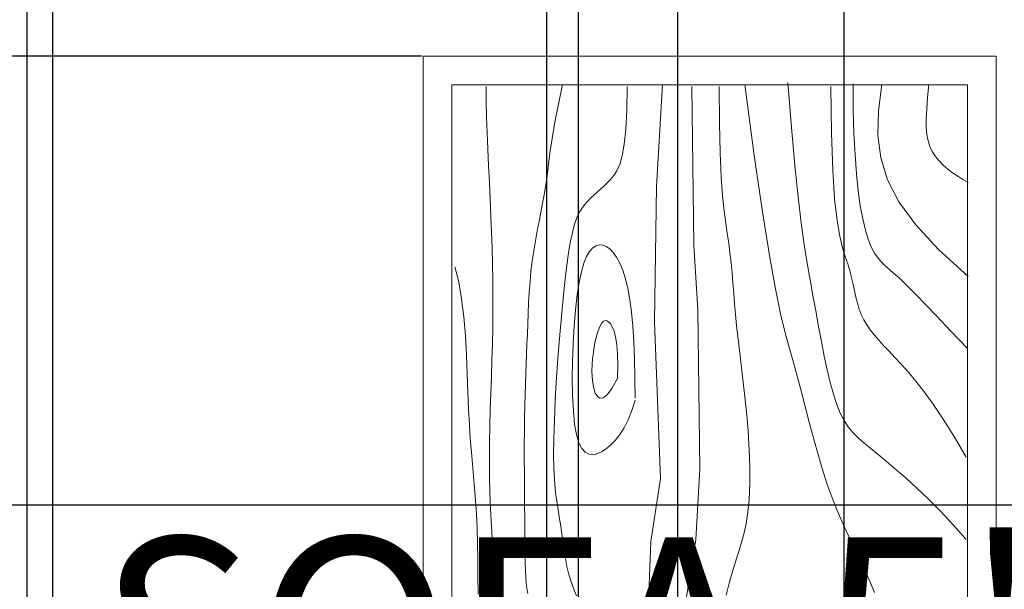
# Model space of a CAD drawing. Units: inches. Extents: x -26 to 385, y 12 to 697.
# Tile 7 of 13: x 223 to 264, y 191 to 215. Entities that reach past the tile are written whole.
import ezdxf

# ---------------------------------------------------------------- set-up
doc = ezdxf.new("R2010")
doc.units = ezdxf.units.IN
doc.header["$MEASUREMENT"] = 0
doc.layers.add('A-ANNO-DIMS', color=4, linetype='Continuous', lineweight=18)
doc.layers.add('Furniture', color=210, linetype='Continuous', lineweight=15)
doc.styles.get("Standard").update_dxf_attribs({"font": 'italic8.shx'})
doc.dimstyles.get("Standard").update_dxf_attribs({"dimtxt": 8, "dimasz": 0.18, "dimexe": 0.18, "dimexo": 0.0625, "dimgap": 0.09, "dimtad": 0, "dimtih": 1, "dimtoh": 1, "dimdec": 4, "dimzin": 0, "dimdsep": 46, "dimlunit": 3, "dimtxsty": 'Standard', "dimcen": 0.09, "dimclrd": 2, "dimclre": 3, "dimclrt": 6, "dimadec": 0, "dimazin": 0, "dimtfac": 1, "dimtdec": 4, "dimtofl": 0, "dimtmove": 0, "dimatfit": 3, "dimfxl": 1, "dimtolj": 1, "dimtzin": 0, "dimarcsym": 0})

# ---------------------------------------------------------------- blocks, each defined once
blk = doc.blocks.new('*D11')
at = {"layer": 'A-ANNO-DIMS', "color": 3, "lineweight": -2, "transparency": 16777216}
for p, q in [((285.56, 224.402), (274.992, 224.402)), ((285.56, 154.738), (274.992, 154.738))]:
    blk.add_line(p, q, dxfattribs=at)
at = {"layer": 'A-ANNO-DIMS', "color": 2, "lineweight": -2, "transparency": 16777216}
for p, q in [((275.172, 224.222), (275.172, 195.755)), ((275.172, 154.918), (275.172, 183.384))]:
    blk.add_line(p, q, dxfattribs=at)
at = {"layer": 'A-ANNO-DIMS', "color": 2, "transparency": 16777216}
for points in [[(275.142, 224.222), (275.202, 224.222), (275.172, 224.402)], [(275.142, 154.918), (275.202, 154.918), (275.172, 154.738)]]:
    blk.add_solid(points, dxfattribs=at)
at = {"layer": 'Defpoints', "color": 0, "transparency": 16777216}
for p in [(285.622, 224.402), (275.172, 154.738), (285.622, 154.738)]:
    blk.add_point(p, dxfattribs=at)
at = {"layer": 'A-ANNO-DIMS', "color": 6, "transparency": 16777216, "insert": (275.172, 189.57), "char_height": 8, "attachment_point": 5}
blk.add_mtext('\\A1;SOFA 5\'-9 1/2" TYP.', dxfattribs=at)
blk = doc.blocks.new('*D28')
at = {"layer": 'A-ANNO-DIMS', "color": 3, "lineweight": -2, "transparency": 16777216}
for p, q in [((141.692, 194.903), (355.559, 194.903)), ((141.692, 158.903), (355.559, 158.903))]:
    blk.add_line(p, q, dxfattribs=at)
at = {"layer": 'A-ANNO-DIMS', "color": 2, "lineweight": -2, "transparency": 16777216}
for p, q in [((355.379, 194.723), (355.379, 181.755)), ((355.379, 159.083), (355.379, 172.052))]:
    blk.add_line(p, q, dxfattribs=at)
at = {"layer": 'A-ANNO-DIMS', "color": 2, "transparency": 16777216}
for points in [[(355.349, 194.723), (355.409, 194.723), (355.379, 194.903)], [(355.349, 159.083), (355.409, 159.083), (355.379, 158.903)]]:
    blk.add_solid(points, dxfattribs=at)
at = {"layer": 'Defpoints', "color": 0, "transparency": 16777216}
for p in [(141.629, 194.903), (355.379, 194.903), (141.629, 158.903)]:
    blk.add_point(p, dxfattribs=at)
at = {"layer": 'A-ANNO-DIMS', "color": 6, "transparency": 16777216, "insert": (355.379, 176.903), "char_height": 8, "attachment_point": 5}
blk.add_mtext('\\A1;3\'-0"', dxfattribs=at)
blk = doc.blocks.new('*D32')
at = {"layer": 'A-ANNO-DIMS', "color": 3, "lineweight": -2, "transparency": 16777216}
for p, q in [((239.825, 213.385), (-5.301, 213.385)), ((239.825, 166.141), (-5.301, 166.141))]:
    blk.add_line(p, q, dxfattribs=at)
at = {"layer": 'A-ANNO-DIMS', "color": 2, "lineweight": -2, "transparency": 16777216}
for p, q in [((-5.121, 213.205), (-5.121, 194.615)), ((-5.121, 166.321), (-5.121, 184.911))]:
    blk.add_line(p, q, dxfattribs=at)
at = {"layer": 'A-ANNO-DIMS', "color": 2, "transparency": 16777216}
for points in [[(-5.151, 213.205), (-5.091, 213.205), (-5.121, 213.385)], [(-5.151, 166.321), (-5.091, 166.321), (-5.121, 166.141)]]:
    blk.add_solid(points, dxfattribs=at)
at = {"layer": 'Defpoints', "color": 0, "transparency": 16777216}
for p in [(-5.121, 213.385), (239.888, 213.385), (239.888, 166.141)]:
    blk.add_point(p, dxfattribs=at)
at = {"layer": 'A-ANNO-DIMS', "color": 6, "transparency": 16777216, "insert": (-5.121, 189.763), "char_height": 8, "attachment_point": 5}
blk.add_mtext('\\A1;3\'-11"', dxfattribs=at)
blk = doc.blocks.new('*D35')
at = {"layer": 'A-ANNO-DIMS', "color": 3, "lineweight": -2, "transparency": 16777216}
for p, q in [((193.598, 147.942), (193.598, 684.809)), ((244.986, 147.942), (244.986, 684.809))]:
    blk.add_line(p, q, dxfattribs=at)
at = {"layer": 'A-ANNO-DIMS', "color": 2, "lineweight": -2, "transparency": 16777216}
for p, q in [((193.778, 684.629), (244.806, 684.629)), ((244.986, 684.629), (245.166, 684.629))]:
    blk.add_line(p, q, dxfattribs=at)
at = {"layer": 'A-ANNO-DIMS', "color": 2, "transparency": 16777216}
for points in [[(193.778, 684.659), (193.778, 684.599), (193.598, 684.629)], [(244.806, 684.659), (244.806, 684.599), (244.986, 684.629)]]:
    blk.add_solid(points, dxfattribs=at)
at = {"layer": 'Defpoints', "color": 0, "transparency": 16777216}
for p in [(244.986, 684.629), (193.598, 147.879), (244.986, 147.879)]:
    blk.add_point(p, dxfattribs=at)
at = {"layer": 'A-ANNO-DIMS', "color": 6, "transparency": 16777216, "insert": (278.398, 684.629), "char_height": 8, "attachment_point": 5}
blk.add_mtext('\\A1;4\'-3 1/2"', dxfattribs=at)
blk = doc.blocks.new('*D36')
at = {"layer": 'A-ANNO-DIMS', "color": 3, "lineweight": -2, "transparency": 16777216}
for p, q in [((146.129, 147.942), (146.129, 684.809)), ((193.598, 147.942), (193.598, 684.809))]:
    blk.add_line(p, q, dxfattribs=at)
at = {"layer": 'A-ANNO-DIMS', "color": 2, "lineweight": -2, "transparency": 16777216}
for p, q in [((146.309, 684.629), (193.418, 684.629)), ((193.598, 684.629), (193.778, 684.629))]:
    blk.add_line(p, q, dxfattribs=at)
at = {"layer": 'A-ANNO-DIMS', "color": 2, "transparency": 16777216}
for points in [[(146.309, 684.659), (146.309, 684.599), (146.129, 684.629)], [(193.418, 684.659), (193.418, 684.599), (193.598, 684.629)]]:
    blk.add_solid(points, dxfattribs=at)
at = {"layer": 'Defpoints', "color": 0, "transparency": 16777216}
for p in [(193.598, 684.629), (146.129, 147.879), (193.598, 147.879)]:
    blk.add_point(p, dxfattribs=at)
at = {"layer": 'A-ANNO-DIMS', "color": 6, "transparency": 16777216, "insert": (228.344, 684.629), "char_height": 8, "attachment_point": 5}
blk.add_mtext('\\A1;3\'-11 1/2"', dxfattribs=at)
blk = doc.blocks.new('*D37')
at = {"layer": 'A-ANNO-DIMS', "color": 3, "lineweight": -2, "transparency": 16777216}
for p, q in [((223.549, 597.317), (223.549, 23.949)), ((257.22, 597.317), (257.22, 23.949))]:
    blk.add_line(p, q, dxfattribs=at)
at = {"layer": 'A-ANNO-DIMS', "color": 2, "lineweight": -2, "transparency": 16777216}
for p, q in [((223.729, 24.129), (257.04, 24.129)), ((257.22, 24.129), (257.4, 24.129))]:
    blk.add_line(p, q, dxfattribs=at)
at = {"layer": 'A-ANNO-DIMS', "color": 2, "transparency": 16777216}
for points in [[(223.729, 24.159), (223.729, 24.099), (223.549, 24.129)], [(257.04, 24.159), (257.04, 24.099), (257.22, 24.129)]]:
    blk.add_solid(points, dxfattribs=at)
at = {"layer": 'Defpoints', "color": 0, "transparency": 16777216}
for p in [(223.549, 597.379), (257.22, 597.379), (257.22, 24.129)]:
    blk.add_point(p, dxfattribs=at)
at = {"layer": 'A-ANNO-DIMS', "color": 6, "transparency": 16777216, "insert": (290.633, 24.129), "char_height": 8, "attachment_point": 5}
blk.add_mtext('\\A1;2\'-9 1/2"', dxfattribs=at)
blk = doc.blocks.new('*D39')
at = {"layer": 'A-ANNO-DIMS', "color": 3, "lineweight": -2, "transparency": 16777216}
for p, q in [((183.359, 597.317), (183.359, 23.949)), ((213.359, 597.317), (213.359, 23.949))]:
    blk.add_line(p, q, dxfattribs=at)
at = {"layer": 'A-ANNO-DIMS', "color": 2, "lineweight": -2, "transparency": 16777216}
for p, q in [((183.539, 24.129), (213.179, 24.129)), ((213.359, 24.129), (213.539, 24.129))]:
    blk.add_line(p, q, dxfattribs=at)
at = {"layer": 'A-ANNO-DIMS', "color": 2, "transparency": 16777216}
for points in [[(183.539, 24.159), (183.539, 24.099), (183.359, 24.129)], [(213.179, 24.159), (213.179, 24.099), (213.359, 24.129)]]:
    blk.add_solid(points, dxfattribs=at)
at = {"layer": 'Defpoints', "color": 0, "transparency": 16777216}
for p in [(183.359, 597.379), (213.359, 597.379), (213.359, 24.129)]:
    blk.add_point(p, dxfattribs=at)
at = {"layer": 'A-ANNO-DIMS', "color": 6, "transparency": 16777216, "insert": (231.533, 24.129), "char_height": 8, "attachment_point": 5}
blk.add_mtext('\\A1;2\'-6"', dxfattribs=at)
blk = doc.blocks.new('*D42')
at = {"layer": 'A-ANNO-DIMS', "color": 3, "lineweight": -2, "transparency": 16777216}
for p, q in [((250.371, 518.992), (250.371, 23.949)), ((274.129, 518.992), (274.129, 23.949))]:
    blk.add_line(p, q, dxfattribs=at)
at = {"layer": 'A-ANNO-DIMS', "color": 2, "lineweight": -2, "transparency": 16777216}
for p, q in [((250.551, 24.129), (273.949, 24.129)), ((274.129, 24.129), (274.309, 24.129))]:
    blk.add_line(p, q, dxfattribs=at)
at = {"layer": 'A-ANNO-DIMS', "color": 2, "transparency": 16777216}
for points in [[(250.551, 24.159), (250.551, 24.099), (250.371, 24.129)], [(273.949, 24.159), (273.949, 24.099), (274.129, 24.129)]]:
    blk.add_solid(points, dxfattribs=at)
at = {"layer": 'Defpoints', "color": 0, "transparency": 16777216}
for p in [(250.371, 519.055), (274.129, 519.055), (274.129, 24.129)]:
    blk.add_point(p, dxfattribs=at)
at = {"layer": 'A-ANNO-DIMS', "color": 6, "transparency": 16777216, "insert": (292.304, 24.129), "char_height": 8, "attachment_point": 5}
blk.add_mtext('\\A1;2\'-0"', dxfattribs=at)
blk = doc.blocks.new('*D46')
at = {"layer": 'A-ANNO-DIMS', "color": 3, "lineweight": -2, "transparency": 16777216}
for p, q in [((224.595, 477.317), (224.595, 23.949)), ((284.629, 477.317), (284.629, 23.949))]:
    blk.add_line(p, q, dxfattribs=at)
at = {"layer": 'A-ANNO-DIMS', "color": 2, "lineweight": -2, "transparency": 16777216}
for p, q in [((224.775, 24.129), (236.617, 24.129)), ((284.449, 24.129), (272.607, 24.129))]:
    blk.add_line(p, q, dxfattribs=at)
at = {"layer": 'A-ANNO-DIMS', "color": 2, "transparency": 16777216}
for points in [[(224.775, 24.159), (224.775, 24.099), (224.595, 24.129)], [(284.449, 24.159), (284.449, 24.099), (284.629, 24.129)]]:
    blk.add_solid(points, dxfattribs=at)
at = {"layer": 'Defpoints', "color": 0, "transparency": 16777216}
for p in [(224.595, 477.379), (284.629, 477.379), (284.629, 24.129)]:
    blk.add_point(p, dxfattribs=at)
at = {"layer": 'A-ANNO-DIMS', "color": 6, "transparency": 16777216, "insert": (254.612, 24.129), "char_height": 8, "attachment_point": 5}
blk.add_mtext('\\A1;5\'-0"', dxfattribs=at)
blk = doc.blocks.new('*D50')
at = {"layer": 'A-ANNO-DIMS', "color": 3, "lineweight": -2, "transparency": 16777216}
for p, q in [((246.278, 401.871), (246.278, 23.949)), ((284.629, 398.317), (284.629, 23.949))]:
    blk.add_line(p, q, dxfattribs=at)
at = {"layer": 'A-ANNO-DIMS', "color": 2, "lineweight": -2, "transparency": 16777216}
for p, q in [((246.458, 24.129), (284.449, 24.129)), ((284.629, 24.129), (284.809, 24.129))]:
    blk.add_line(p, q, dxfattribs=at)
at = {"layer": 'A-ANNO-DIMS', "color": 2, "transparency": 16777216}
for points in [[(246.458, 24.159), (246.458, 24.099), (246.278, 24.129)], [(284.449, 24.159), (284.449, 24.099), (284.629, 24.129)]]:
    blk.add_solid(points, dxfattribs=at)
at = {"layer": 'Defpoints', "color": 0, "transparency": 16777216}
for p in [(246.278, 401.934), (284.629, 398.379), (284.629, 24.129)]:
    blk.add_point(p, dxfattribs=at)
at = {"layer": 'A-ANNO-DIMS', "color": 6, "transparency": 16777216, "insert": (318.042, 24.129), "char_height": 8, "attachment_point": 5}
blk.add_mtext('\\A1;3\'-2 1/2"', dxfattribs=at)

msp = doc.modelspace()

# ---------------------------------------------------------------- linework, layer by layer
at = {"layer": 'Furniture'}
for p, q in [((239.88756, 166.14113), (239.88756, 213.38513)), ((239.88756, 213.38513), (263.50956, 213.38513)), ((263.50956, 213.38513), (263.50956, 166.14113)), ((254.91435, 212.30259), (255.06209, 210.44149)), ((241.06866, 167.32223), (241.06866, 212.20403)), ((241.06866, 212.20403), (262.32846, 212.20403)), ((242.4795, 212.14102), (242.48485, 211.52259)), ((245.62858, 212.2218), (245.44175, 211.33552)), ((248.29319, 212.14102), (248.27861, 211.15771)), ((249.74662, 212.2218), (249.50438, 208.0209)), ((250.9578, 212.14102), (251.03855, 205.5973)), ((252.08825, 212.14102), (252.09894, 210.63069)), ((253.13794, 212.2218), (253.53101, 209.28852)), ((256.69075, 212.14102), (256.71032, 210.21153)), ((257.60587, 212.24873), (257.61514, 211.18493)), ((258.79014, 212.2218), (258.65467, 211.12945)), ((260.72804, 212.2218), (260.67533, 211.68458)), ((262.32846, 212.20403), (262.32846, 167.32223)), ((242.48485, 211.52259), (242.49958, 210.88199)), ((260.67533, 211.68458), (260.63941, 211.2186)), ((245.44175, 211.33552), (245.29971, 210.59976)), ((248.27861, 211.15771), (248.23705, 210.37139)), ((257.61514, 211.18493), (257.64215, 210.21382)), ((258.65467, 211.12945), (258.62991, 210.13271)), ((260.63941, 211.2186), (260.62195, 210.81557)), ((242.49958, 210.88199), (242.52172, 210.22356)), ((260.62195, 210.81557), (260.62459, 210.46722)), ((245.29971, 210.59976), (245.19426, 209.99086)), ((248.23705, 210.37139), (248.17184, 209.75564)), ((252.09894, 210.63069), (252.12841, 209.40437)), ((255.06209, 210.44149), (255.20306, 208.88799)), ((260.62459, 210.46722), (260.64899, 210.16526)), ((242.52172, 210.22356), (242.54931, 209.55164)), ((245.19426, 209.99086), (245.11719, 209.48516)), ((256.71032, 210.21153), (256.76404, 208.68676)), ((257.64215, 210.21382), (257.68571, 209.33343)), ((258.62991, 210.13271), (258.74331, 209.19846)), ((260.64899, 210.16526), (260.69682, 209.9014)), ((260.69682, 209.9014), (260.76972, 209.66736)), ((242.54931, 209.55164), (242.58037, 208.87057)), ((245.11719, 209.48516), (245.06031, 209.05898)), ((248.17184, 209.75564), (248.08628, 209.28403)), ((260.76972, 209.66736), (260.86935, 209.45486)), ((260.86935, 209.45486), (260.99642, 209.25688)), ((245.06031, 209.05898), (245.01542, 208.68865)), ((248.08628, 209.28403), (247.9837, 208.93013)), ((252.12841, 209.40437), (252.1727, 208.42042)), ((253.53101, 209.28852), (253.8677, 206.97036)), ((257.68571, 209.33343), (257.74465, 208.54181)), ((258.74331, 209.19846), (259.02229, 208.29356)), ((260.99642, 209.25688), (261.14786, 209.07144)), ((261.14786, 209.07144), (261.31964, 208.89784)), ((242.58037, 208.87057), (242.61292, 208.18468)), ((245.01542, 208.68865), (244.97431, 208.35052)), ((247.86739, 208.66751), (247.74067, 208.46974)), ((247.9837, 208.93013), (247.86739, 208.66751)), ((255.20306, 208.88799), (255.33803, 207.59752)), ((256.76404, 208.68676), (256.8444, 207.50944)), ((261.31964, 208.89784), (261.50774, 208.73536)), ((261.50774, 208.73536), (261.70815, 208.58329)), ((244.97431, 208.35052), (244.92879, 208.0209)), ((247.60686, 208.31039), (247.46897, 208.16697)), ((247.74067, 208.46974), (247.60686, 208.31039)), ((252.1727, 208.42042), (252.22787, 207.63717)), ((257.74465, 208.54181), (257.81779, 207.83696)), ((259.02229, 208.29356), (259.4943, 207.38487)), ((261.70815, 208.58329), (261.91683, 208.44093)), ((261.91683, 208.44093), (262.12978, 208.30756)), ((262.12978, 208.30756), (262.34296, 208.18248)), ((242.61292, 208.18468), (242.645, 207.49833)), ((244.92879, 208.0209), (244.87251, 207.68024)), ((247.18814, 207.90507), (247.04836, 207.78107)), ((247.32887, 208.03279), (247.18814, 207.90507)), ((247.46897, 208.16697), (247.32887, 208.03279)), ((249.50438, 208.0209), (249.42364, 202.44663)), ((257.81779, 207.83696), (257.90394, 207.21693)), ((242.645, 207.49833), (242.67463, 206.81584)), ((244.87251, 207.68024), (244.80662, 207.32538)), ((246.77795, 207.53313), (246.65047, 207.40368)), ((246.91111, 207.65801), (246.77795, 207.53313)), ((247.04836, 207.78107), (246.91111, 207.65801)), ((252.22787, 207.63717), (252.28998, 207.01296)), ((255.33803, 207.59752), (255.46779, 206.52551)), ((256.8444, 207.50944), (256.94393, 206.62228)), ((244.80662, 207.32538), (244.7341, 206.95726)), ((246.41838, 207.11802), (246.31408, 206.94438)), ((246.53025, 207.26689), (246.41838, 207.11802)), ((246.65047, 207.40368), (246.53025, 207.26689)), ((252.28998, 207.01296), (252.35508, 206.50615)), ((257.90394, 207.21693), (258.00191, 206.67973)), ((259.4943, 207.38487), (260.18679, 206.43925)), ((242.67463, 206.81584), (242.70014, 206.14058)), ((244.7341, 206.95726), (244.65795, 206.57684)), ((246.21609, 206.73129), (246.12315, 206.46408)), ((246.31408, 206.94438), (246.21609, 206.73129)), ((253.8677, 206.97036), (254.15598, 205.17432)), ((256.94393, 206.62228), (257.05512, 205.96802)), ((258.00191, 206.67973), (258.11053, 206.2234)), ((244.65795, 206.57684), (244.58118, 206.18506)), ((246.12315, 206.46408), (246.03399, 206.12807)), ((252.35508, 206.50615), (252.41925, 206.07508)), ((255.46779, 206.52551), (255.59314, 205.62738)), ((258.11053, 206.2234), (258.22875, 205.84438)), ((260.18679, 206.43925), (261.1272, 205.42358)), ((242.70014, 206.14058), (242.721, 205.47202)), ((244.58118, 206.18506), (244.50676, 205.78286)), ((246.03399, 206.12807), (245.94736, 205.7086)), ((252.41925, 206.07508), (252.47852, 205.67809)), ((257.05512, 205.96802), (257.1705, 205.48938)), ((258.22875, 205.84438), (258.35603, 205.53282)), ((242.721, 205.47202), (242.73697, 204.80867)), ((244.50676, 205.78286), (244.43772, 205.3712)), ((245.94736, 205.7086), (245.86199, 205.19098)), ((246.86437, 205.48391), (246.73818, 205.33882)), ((246.99719, 205.57251), (246.86437, 205.48391)), ((247.13584, 205.61077), (246.99719, 205.57251)), ((247.27926, 205.60363), (247.13584, 205.61077)), ((247.42528, 205.55113), (247.27926, 205.60363)), ((247.57146, 205.45207), (247.42528, 205.55113)), ((247.71536, 205.30529), (247.57146, 205.45207)), ((251.03855, 205.5973), (251.20004, 202.93135)), ((252.47852, 205.67809), (252.52993, 205.2805)), ((255.59314, 205.62738), (255.71487, 204.85855)), ((257.1705, 205.48938), (257.28256, 205.12907)), ((258.35603, 205.53282), (258.49199, 205.27727)), ((261.1272, 205.42358), (262.34296, 204.30472)), ((244.43772, 205.3712), (244.37702, 204.95101)), ((245.86199, 205.19098), (245.77662, 204.56054)), ((246.6194, 205.1311), (246.50882, 204.85458)), ((246.73818, 205.33882), (246.6194, 205.1311)), ((247.85452, 205.1096), (247.71536, 205.30529)), ((247.98651, 204.86381), (247.85452, 205.1096)), ((252.52993, 205.2805), (252.5744, 204.87548)), ((254.15598, 205.17432), (254.4038, 203.80738)), ((257.28256, 205.12907), (257.38382, 204.82983)), ((258.49199, 205.27727), (258.63622, 205.0663)), ((258.63622, 205.0663), (258.78834, 204.88846)), ((241.18757, 204.70865), (241.34764, 204.08917)), ((242.73697, 204.80867), (242.74781, 204.14904)), ((244.37702, 204.95101), (244.32693, 204.52349)), ((246.50882, 204.85458), (246.40723, 204.50311)), ((248.10887, 204.56674), (247.98651, 204.86381)), ((252.5744, 204.87548), (252.61383, 204.46321)), ((255.71487, 204.85855), (255.83375, 204.17445)), ((257.38382, 204.82983), (257.46881, 204.54411)), ((258.78834, 204.88846), (258.94796, 204.73232)), ((258.94796, 204.73232), (259.11466, 204.58643)), ((259.11466, 204.58643), (259.28808, 204.43936)), ((244.32693, 204.52349), (244.28661, 204.09076)), ((245.77662, 204.56054), (245.69062, 203.81027)), ((246.40723, 204.50311), (246.31542, 204.07054)), ((248.21918, 204.2172), (248.10887, 204.56674)), ((248.31544, 203.81383), (248.21918, 204.2172)), ((252.61383, 204.46321), (252.6501, 204.04385)), ((255.83375, 204.17445), (255.95058, 203.53051)), ((257.46881, 204.54411), (257.54016, 204.26327)), ((257.54016, 204.26327), (257.60252, 203.98844)), ((259.28808, 204.43936), (259.47062, 204.27868)), ((259.47062, 204.27868), (259.67603, 204.08803)), ((241.34764, 204.08917), (241.46892, 203.39576)), ((242.74781, 204.14904), (242.75329, 203.49161)), ((244.28661, 204.09076), (244.25449, 203.65519)), ((245.69062, 203.81027), (245.60587, 202.96375)), ((246.31542, 204.07054), (246.23418, 203.55071)), ((248.3976, 203.35453), (248.31544, 203.81383)), ((252.6501, 204.04385), (252.68511, 203.61753)), ((254.4038, 203.80738), (254.61913, 202.77652)), ((257.60252, 203.98844), (257.66054, 203.7207)), ((259.67603, 204.08803), (259.92087, 203.85003)), ((259.92087, 203.85003), (260.2217, 203.54734)), ((241.46892, 203.39576), (241.55802, 202.64919)), ((242.75329, 203.49161), (242.75317, 202.83489)), ((244.25449, 203.65519), (244.22899, 203.21915)), ((246.23418, 203.55071), (246.16442, 202.94279)), ((252.68511, 203.61753), (252.72075, 203.18444)), ((255.95058, 203.53051), (256.06621, 202.89107)), ((257.66054, 203.7207), (257.71888, 203.46117)), ((257.71888, 203.46117), (257.78219, 203.21094)), ((260.2217, 203.54734), (260.59507, 203.16261)), ((244.22899, 203.21915), (244.20854, 202.785)), ((245.60587, 202.96375), (245.52492, 202.05221)), ((248.46603, 202.837), (248.3976, 203.35453)), ((252.72075, 203.18444), (252.75892, 202.74471)), ((257.78219, 203.21094), (257.85511, 202.97113)), ((257.85511, 202.97113), (257.94231, 202.74284)), ((260.59507, 203.16261), (261.05754, 202.67847)), ((241.55802, 202.64919), (241.62158, 201.87018)), ((242.75317, 202.83489), (242.74722, 202.17738)), ((244.20854, 202.785), (244.19156, 202.35511)), ((246.16442, 202.94279), (246.10759, 202.26717)), ((248.52113, 202.25897), (248.46603, 202.837)), ((251.20004, 202.93135), (251.28079, 196.38763)), ((252.75892, 202.74471), (252.8015, 202.29852)), ((254.61913, 202.77652), (254.80995, 201.98873)), ((256.06621, 202.89107), (256.18168, 202.25613)), ((257.94231, 202.74284), (258.04769, 202.52623)), ((261.05754, 202.67847), (261.62568, 202.07756)), ((242.74722, 202.17738), (242.73519, 201.51758)), ((244.19156, 202.35511), (244.17647, 201.93185)), ((246.10759, 202.26717), (246.06527, 201.54959)), ((247.13437, 202.18533), (247.07993, 202.03317)), ((247.19164, 202.30909), (247.13437, 202.18533)), ((247.25191, 202.40287), (247.19164, 202.30909)), ((247.31533, 202.46509), (247.25191, 202.40287)), ((247.38207, 202.49417), (247.31533, 202.46509)), ((247.45228, 202.48855), (247.38207, 202.49417)), ((247.52611, 202.44663), (247.45228, 202.48855)), ((247.60299, 202.36584), (247.52611, 202.44663)), ((247.6794, 202.23961), (247.60299, 202.36584)), ((247.75108, 202.06037), (247.6794, 202.23961)), ((248.56331, 201.61813), (248.52113, 202.25897)), ((249.42364, 202.44663), (249.66587, 195.9837)), ((252.8015, 202.29852), (252.84981, 201.84591)), ((256.18168, 202.25613), (256.29809, 201.63459)), ((258.04769, 202.52623), (258.17214, 202.31766)), ((258.17214, 202.31766), (258.31584, 202.11257)), ((241.62158, 201.87018), (241.66621, 201.0795)), ((244.17647, 201.93185), (244.1617, 201.51758)), ((245.52492, 202.05221), (245.45027, 201.10692)), ((247.02818, 201.85419), (246.9793, 201.65052)), ((247.07993, 202.03317), (247.02818, 201.85419)), ((247.81377, 201.82053), (247.75108, 202.06037)), ((247.86321, 201.51253), (247.81377, 201.82053)), ((252.84981, 201.84591), (252.90285, 201.38651)), ((254.80995, 201.98873), (254.9842, 201.351)), ((258.31584, 202.11257), (258.47894, 201.90637)), ((258.47894, 201.90637), (258.66159, 201.69449)), ((261.62568, 202.07756), (262.31604, 201.34254)), ((242.73519, 201.51758), (242.71729, 200.85425)), ((244.1617, 201.51758), (244.14604, 201.11304)), ((246.06527, 201.54959), (246.03904, 200.81575)), ((246.93492, 201.42649), (246.897, 201.18699)), ((246.9793, 201.65052), (246.93492, 201.42649)), ((247.89514, 201.1288), (247.86321, 201.51253)), ((248.59294, 200.91221), (248.56331, 201.61813)), ((252.90285, 201.38651), (252.95905, 200.91986)), ((254.9842, 201.351), (255.14986, 200.77031)), ((256.29809, 201.63459), (256.41655, 201.03539)), ((258.66159, 201.69449), (258.86395, 201.47235)), ((258.86395, 201.47235), (259.08619, 201.23538)), ((241.66621, 201.0795), (241.69854, 200.29789)), ((244.14604, 201.11304), (244.12974, 200.71245)), ((245.45027, 201.10692), (245.38445, 200.15909)), ((246.86753, 200.93693), (246.84846, 200.68118)), ((246.897, 201.18699), (246.86753, 200.93693)), ((247.90531, 200.66175), (247.89514, 201.1288)), ((256.41655, 201.03539), (256.53817, 200.46742)), ((259.08619, 201.23538), (259.32845, 200.979)), ((259.32845, 200.979), (259.5914, 200.69707)), ((242.71729, 200.85425), (242.69545, 200.18713)), ((244.12974, 200.71245), (244.11344, 200.30839)), ((246.03904, 200.81575), (246.03047, 200.09138)), ((246.84846, 200.68118), (246.84177, 200.42465)), ((247.88947, 200.10382), (247.90531, 200.66175)), ((248.61043, 200.13891), (248.59294, 200.91221)), ((252.95905, 200.91986), (253.01682, 200.44548)), ((255.14986, 200.77031), (255.31373, 200.17076)), ((259.5914, 200.69707), (259.87769, 200.3771)), ((241.69854, 200.29789), (241.72519, 199.54611)), ((242.69545, 200.18713), (242.67203, 199.51622)), ((244.11344, 200.30839), (244.09778, 199.89343)), ((245.38445, 200.15909), (245.32999, 199.23999)), ((246.84177, 200.42465), (246.84943, 200.17222)), ((246.84943, 200.17222), (246.87341, 199.92878)), ((248.61618, 199.29595), (248.61043, 200.13891)), ((253.01682, 200.44548), (253.07459, 199.96289)), ((255.31373, 200.17076), (255.47799, 199.54494)), ((256.53817, 200.46742), (256.66405, 199.93961)), ((259.87769, 200.3771), (260.19047, 200.00507)), ((244.09778, 199.89343), (244.08337, 199.46018)), ((246.03047, 200.09138), (246.04114, 199.40219)), ((246.87341, 199.92878), (246.91569, 199.70159)), ((247.66393, 199.69923), (247.88947, 200.10382)), ((253.07459, 199.96289), (253.13079, 199.47162)), ((256.66405, 199.93961), (256.79529, 199.46088)), ((260.19047, 200.00507), (260.53291, 199.56692)), ((241.72519, 199.54611), (241.75279, 198.84489)), ((242.67203, 199.51622), (242.6494, 198.84153)), ((244.08337, 199.46018), (244.07086, 199.0012)), ((246.04114, 199.40219), (246.07263, 198.77391)), ((246.91569, 199.70159), (246.97824, 199.50738)), ((246.97824, 199.50738), (247.06302, 199.36524)), ((247.06302, 199.36524), (247.17201, 199.29427)), ((247.17201, 199.29427), (247.30717, 199.31354)), ((247.30717, 199.31354), (247.47049, 199.44217)), ((247.47049, 199.44217), (247.66393, 199.69923)), ((253.13079, 199.47162), (253.18383, 198.9712)), ((255.47799, 199.54494), (255.64367, 198.90255)), ((256.79529, 199.46088), (256.93299, 199.04013)), ((260.53291, 199.56692), (260.90814, 199.04862)), ((244.07086, 199.0012), (244.06088, 198.5091)), ((245.32999, 199.23999), (245.28941, 198.38084)), ((248.48431, 198.78688), (248.61618, 199.21516)), ((253.18383, 198.9712), (253.23214, 198.46115)), ((255.64367, 198.90255), (255.8118, 198.2533)), ((256.93299, 199.04013), (257.07874, 198.68265)), ((260.90814, 199.04862), (261.31934, 198.43612)), ((241.75279, 198.84489), (241.78654, 198.20913)), ((242.6494, 198.84153), (242.62992, 198.16304)), ((244.06088, 198.5091), (244.05404, 197.97644)), ((246.07263, 198.77391), (246.12652, 198.23226)), ((248.33336, 198.4094), (248.48431, 198.78688)), ((257.07874, 198.68265), (257.236, 198.37921)), ((241.78654, 198.20913), (241.82596, 197.63025)), ((242.62992, 198.16304), (242.61597, 197.48078)), ((245.28941, 198.38084), (245.26523, 197.6129)), ((246.12652, 198.23226), (246.20374, 197.79706)), ((248.16695, 198.08052), (248.33336, 198.4094)), ((253.23214, 198.46115), (253.27415, 197.94206)), ((255.8118, 198.2533), (255.9834, 197.60689)), ((257.236, 198.37921), (257.40871, 198.11696)), ((257.40871, 198.11696), (257.60083, 197.88303)), ((261.31934, 198.43612), (261.76964, 197.71538)), ((244.05404, 197.97644), (244.05078, 197.39957)), ((246.20374, 197.79706), (246.30273, 197.46458)), ((247.80228, 197.55972), (247.98872, 197.79803)), ((247.98872, 197.79803), (248.16695, 198.08052)), ((253.27415, 197.94206), (253.30826, 197.41871)), ((257.60083, 197.88303), (257.81628, 197.66456)), ((261.76964, 197.71538), (262.26221, 196.87235)), ((241.82596, 197.63025), (241.86917, 197.09382)), ((242.61597, 197.48078), (242.6099, 196.79472)), ((244.05078, 197.39957), (244.05068, 196.78988)), ((245.26523, 197.6129), (245.25908, 196.95924)), ((246.30273, 197.46458), (246.42127, 197.22519)), ((247.41932, 197.20681), (247.61127, 197.36338)), ((247.61127, 197.36338), (247.80228, 197.55972)), ((253.30826, 197.41871), (253.33292, 196.89694)), ((255.9834, 197.60689), (256.15949, 196.97302)), ((257.81628, 197.66456), (258.05902, 197.44869)), ((258.05902, 197.44869), (258.33298, 197.22257)), ((241.86917, 197.09382), (241.91428, 196.58539)), ((245.25908, 196.95924), (245.26901, 196.41035)), ((246.42127, 197.22519), (246.55716, 197.06927)), ((246.55716, 197.06927), (246.70819, 196.98719)), ((246.70819, 196.98719), (246.87215, 196.96934)), ((246.87215, 196.96934), (247.04684, 197.00608)), ((247.04684, 197.00608), (247.23004, 197.08778)), ((247.23004, 197.08778), (247.41932, 197.20681)), ((253.33292, 196.89694), (253.34653, 196.38258)), ((256.15949, 196.97302), (256.34111, 196.3614)), ((258.33298, 197.22257), (258.64211, 196.97334)), ((258.64211, 196.97334), (258.9892, 196.68983)), ((241.91428, 196.58539), (241.95938, 196.09053)), ((242.6099, 196.79472), (242.61408, 196.10488)), ((244.05068, 196.78988), (244.0531, 196.16252)), ((258.9892, 196.68983), (259.3724, 196.36775)), ((241.95938, 196.09053), (242.00259, 195.59481)), ((242.61408, 196.10488), (242.63024, 195.41117)), ((244.0531, 196.16252), (244.05741, 195.53264)), ((245.26901, 196.41035), (245.2922, 195.94857)), ((251.28079, 196.38763), (251.1193, 193.47931)), ((253.34653, 196.38258), (253.34753, 195.88148)), ((256.34111, 196.3614), (256.52926, 195.78173)), ((259.3724, 196.36775), (259.78872, 196.00449)), ((245.2922, 195.94857), (245.32579, 195.5562)), ((249.66587, 195.9837), (249.26214, 193.39853)), ((253.34753, 195.88148), (253.33434, 195.39947)), ((256.52926, 195.78173), (256.72448, 195.24113)), ((259.78872, 196.00449), (260.23516, 195.59744)), ((242.00259, 195.59481), (242.04202, 195.08378)), ((242.63024, 195.41117), (242.6576, 194.7132)), ((244.05741, 195.53264), (244.06298, 194.91538)), ((245.32579, 195.5562), (245.36695, 195.2156)), ((253.33434, 195.39947), (253.30537, 194.94239)), ((260.23516, 195.59744), (260.70872, 195.144)), ((242.04202, 195.08378), (242.07577, 194.54301)), ((244.06298, 194.91538), (244.06918, 194.32589)), ((245.36695, 195.2156), (245.41284, 194.90907)), ((245.41284, 194.90907), (245.46063, 194.61895)), ((253.30537, 194.94239), (253.25906, 194.51608)), ((256.72448, 195.24113), (256.92521, 194.73635)), ((260.70872, 195.144), (261.20642, 194.64157)), ((242.07577, 194.54301), (242.10234, 193.96075)), ((242.6576, 194.7132), (242.69474, 194.0105)), ((245.46063, 194.61895), (245.50747, 194.32757)), ((253.25906, 194.51608), (253.19461, 194.12385)), ((256.92521, 194.73635), (257.12941, 194.26154)), ((261.20642, 194.64157), (261.72525, 194.08754)), ((244.06918, 194.32589), (244.07538, 193.77932)), ((245.50747, 194.32757), (245.55144, 194.02097)), ((253.19461, 194.12385), (253.11439, 193.75891)), ((257.12941, 194.26154), (257.33504, 193.81088)), ((261.72525, 194.08754), (262.26221, 193.47931)), ((242.10234, 193.96075), (242.12182, 193.33604)), ((242.69474, 194.0105), (242.74024, 193.30259)), ((244.07538, 193.77932), (244.08096, 193.29081)), ((245.55144, 194.02097), (245.59431, 193.70001)), ((245.59431, 193.70001), (245.63876, 193.36926)), ((253.11439, 193.75891), (253.02155, 193.41197)), ((257.33504, 193.81088), (257.54003, 193.37852)), ((242.12182, 193.33604), (242.13467, 192.67063)), ((242.74024, 193.30259), (242.79268, 192.58901)), ((244.08096, 193.29081), (244.08571, 192.8711)), ((245.63876, 193.36926), (245.68746, 193.03331)), ((249.26214, 193.39853), (249.10065, 188.87448)), ((251.1193, 193.47931), (250.63482, 190.49021)), ((253.02155, 193.41197), (252.91925, 193.0737)), ((257.54003, 193.37852), (257.74234, 192.95862)), ((244.08571, 192.8711), (244.09126, 192.51324)), ((245.68746, 193.03331), (245.74311, 192.69672)), ((252.91925, 193.0737), (252.81065, 192.7348)), ((257.74234, 192.95862), (257.93992, 192.54535)), ((242.13467, 192.67063), (242.14138, 191.96625)), ((242.79268, 192.58901), (242.85064, 191.86926)), ((244.09126, 192.51324), (244.09964, 192.20587)), ((245.74311, 192.69672), (245.80837, 192.36408)), ((252.81065, 192.7348), (252.69889, 192.38596)), ((257.93992, 192.54535), (258.13072, 192.13287)), ((244.09964, 192.20587), (244.11292, 191.93764)), ((245.80837, 192.36408), (245.88593, 192.03996)), ((245.88593, 192.03996), (245.97848, 191.72894)), ((252.58712, 192.01787), (252.47852, 191.62122)), ((252.69889, 192.38596), (252.58712, 192.01787)), ((258.13072, 192.13287), (258.31298, 191.71684)), ((242.14138, 191.96625), (242.1424, 191.22463)), ((242.85064, 191.86926), (242.91269, 191.14289)), ((244.11292, 191.93764), (244.13313, 191.69717)), ((244.13313, 191.69717), (244.16233, 191.47311)), ((245.97848, 191.72894), (246.08743, 191.4343)), ((252.47852, 191.62122), (252.37572, 191.18868)), ((258.31298, 191.71684), (258.48609, 191.29892)), ((244.16233, 191.47311), (244.20257, 191.25411)), ((246.08743, 191.4343), (246.20915, 191.15418))]:
    msp.add_line(p, q, dxfattribs=at)

# ---------------------------------------------------------------- dimensions: what is measured, and where the dimension line sits
at = {"layer": 'A-ANNO-DIMS'}
for base, p1, p2, picture, middle in [((193.59818, 684.62909), (146.12932, 147.87909), (193.59818, 147.87909), '*D36', (228.34437, 684.62909)), ((244.98557, 684.62909), (193.59818, 147.87909), (244.98557, 147.87909), '*D35', (278.39843, 684.62909)), ((213.35855, 24.12909), (183.35855, 597.37909), (213.35855, 597.37909), '*D39', (231.53331, 24.12909)), ((257.21981, 24.12909), (223.54856, 597.37909), (257.21981, 597.37909), '*D37', (290.63267, 24.12909)), ((274.12932, 24.12909), (250.37102, 519.05498), (274.12932, 519.05498), '*D42', (292.30408, 24.12909)), ((284.62932, 24.12909), (224.59493, 477.37909), (284.62932, 477.37909), '*D46', (254.61213, 24.12909)), ((284.62932, 24.12909), (246.27828, 401.934), (284.62932, 398.37909), '*D50', (318.04218, 24.12909))]:
    dim = msp.add_linear_dim(base=base, p1=p1, p2=p2, dimstyle='Standard', override={"dimdec": 1, "dimlfac": 1, "dimrnd": 0, "dimzin": 1, "dimdsep": 46, "dimlunit": 4, "dimfrac": 2}, dxfattribs=at)
    dim.commit()
    dim.dimension.update_dxf_attribs({"geometry": picture, "text_midpoint": middle})
dim = msp.add_linear_dim(base=(275.17245, 154.73754), p1=(285.62207, 224.40165), p2=(285.62207, 154.73754), angle=270, text='SOFA <> TYP.', dimstyle='Standard', override={"dimdec": 1, "dimlfac": 1, "dimrnd": 0, "dimzin": 1, "dimdsep": 46, "dimlunit": 4, "dimfrac": 2}, dxfattribs=at)
dim.commit()
dim.dimension.update_dxf_attribs({"geometry": '*D11', "text_midpoint": (275.17245, 189.56959)})
for base, p1, p2, picture, middle in [((-5.12068, 213.38513), (239.88756, 166.14113), (239.88756, 213.38513), '*D32', (-5.12068, 189.76313)), ((355.37932, 194.90341), (141.62932, 158.90341), (141.62932, 194.90341), '*D28', (355.37932, 176.90341))]:
    dim = msp.add_linear_dim(base=base, p1=p1, p2=p2, angle=90, dimstyle='Standard', override={"dimdec": 1, "dimlfac": 1, "dimrnd": 0, "dimzin": 1, "dimdsep": 46, "dimlunit": 4, "dimfrac": 2}, dxfattribs=at)
    dim.commit()
    dim.dimension.update_dxf_attribs({"geometry": picture, "text_midpoint": middle})

doc.saveas('drawing.dxf')
